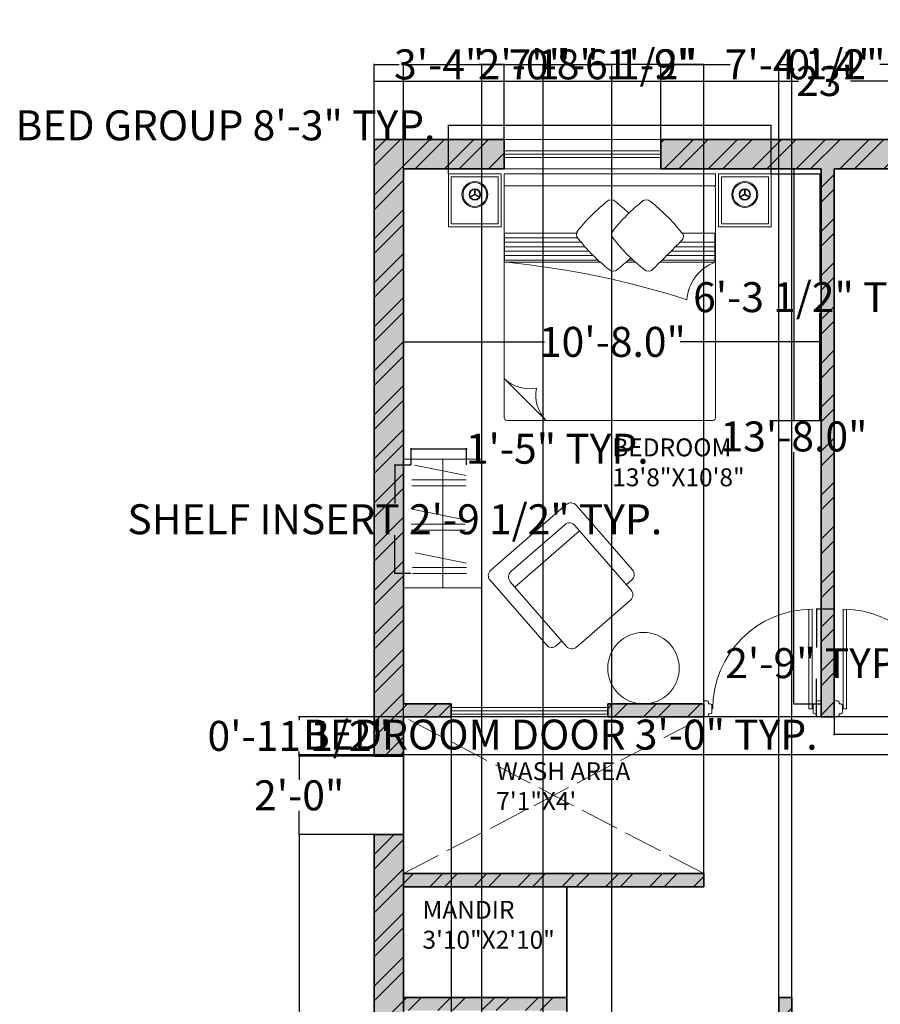
# Model space of a CAD drawing. Units: inches. Extents: x 1086 to 1540, y 3343 to 3848.
# Tile 3 of 8: x 1086 to 1350, y 3547 to 3848. Entities that reach past the tile are written whole.
import ezdxf

# ---------------------------------------------------------------- set-up
doc = ezdxf.new("R2010")
doc.units = ezdxf.units.IN
doc.linetypes.add('ACAD_ISO02W100', pattern=[15, 12, -3])
for name, color, linetype, lineweight in [('00 FURNITURE', 15, 'Continuous', 15), ('A-ANNO-DIMS', 2, 'Continuous', 13), ('A-AREA-IDEN', 7, 'Continuous', 18), ('A-DOOR', 4, 'Continuous', 20), ('A-FLOR-CASE', 8, 'Continuous', 18), ('A-FLOR-OPEN', 8, 'ACAD_ISO02W100', 13), ('A-WALL-PATT', 252, 'Continuous', 9), ('WALL', 7, 'Continuous', 35), ('WINDOW', 160, 'Continuous', 15)]:
    doc.layers.add(name, color=color, linetype=linetype, lineweight=lineweight)
doc.styles.get("Standard").update_dxf_attribs({"font": 'arial.ttf'})
doc.dimstyles.get("Standard").update_dxf_attribs({"dimtxt": 9.18, "dimasz": 0.18, "dimexe": 0.18, "dimexo": 0.0625, "dimgap": 0.09, "dimtad": 0, "dimtih": 1, "dimtoh": 1, "dimdec": 1, "dimzin": 0, "dimdsep": 46, "dimlunit": 3, "dimtxsty": 'Standard', "dimcen": 0.09, "dimadec": 0, "dimazin": 0, "dimtfac": 1, "dimtdec": 1, "dimtofl": 0, "dimtmove": 0, "dimatfit": 3, "dimfxl": 1, "dimtolj": 1, "dimtzin": 0, "dimarcsym": 0})

# ---------------------------------------------------------------- blocks, each defined once
blk = doc.blocks.new('DDD')
at = {"layer": '00 FURNITURE'}
for p, q in [((-12579.77, -15859.53), (-12579.77, -15829.05)), ((-12578.77, -15859.53), (-12578.77, -15829.03)), ((-12612.02, -15857.03), (-12612.02, -15862.03)), ((-12611.02, -15857.03), (-12612.02, -15857.03)), ((-12610.52, -15858.03), (-12610.52, -15857.53)), ((-12578.77, -15859.53), (-12579.77, -15859.53)), ((-12577.52, -15858.03), (-12577.52, -15857.53)), ((-12577.02, -15857.03), (-12576.02, -15857.03)), ((-12576.02, -15857.03), (-12576.02, -15862.03)), ((-12612.02, -15862.03), (-12611.02, -15862.03)), ((-12610.52, -15861.53), (-12610.52, -15861.03)), ((-12577.52, -15861.53), (-12577.52, -15861.03)), ((-12576.02, -15862.03), (-12577.02, -15862.03))]:
    blk.add_line(p, q, dxfattribs=at)
for points in [[(-12610.52, -15861.03), (-12610.02, -15861.03, 0.414214), (-12609.52, -15860.53), (-12609.52, -15858.53, 0.414214), (-12610.02, -15858.03), (-12610.52, -15858.03)], [(-12577.52, -15861.03), (-12578.02, -15861.03, -0.414214), (-12578.52, -15860.53), (-12578.52, -15858.53, -0.414214), (-12578.02, -15858.03), (-12577.52, -15858.03)]]:
    blk.add_lwpolyline(points, format="xyb", dxfattribs=at)
for centre, radius, start, end in [((-12578.77, -15859.53), 30.5, 90, 180), ((-12611.02, -15857.53), 0.5, 0, 90), ((-12577.02, -15857.53), 0.5, 90, 180), ((-12611.02, -15861.53), 0.5, 270, 0), ((-12577.02, -15861.53), 0.5, 180, 270)]:
    blk.add_arc(centre, radius, start, end, dxfattribs=at)
blk = doc.blocks.new('RGWTG')
at = {"layer": '00 FURNITURE'}
for p, q in [((578.23, 3473.51), (577.36, 3475.01)), ((578.23, 3473.58), (577.36, 3472.08)), ((578.36, 3473.58), (577.49, 3475.09)), ((578.36, 3473.51), (577.49, 3472)), ((578.29, 3473.62), (580.03, 3473.62)), ((578.29, 3473.47), (580.03, 3473.47)), ((521.93, 3464.58), (509.03, 3451.68)), ((509.93, 3464.58), (566.4, 3464.58)), ((557.53, 3463.84), (557.53, 3464.49)), ((557.53, 3464.49), (566.4, 3464.49)), ((558.2, 3464.49), (558.2, 3435.82)), ((559.57, 3464.49), (559.57, 3437.25)), ((560.94, 3464.49), (560.94, 3438.58)), ((562.3, 3464.49), (562.3, 3439.83)), ((563.67, 3464.49), (563.67, 3440.99)), ((565.04, 3464.49), (565.04, 3442.08)), ((566.4, 3464.58), (580.98, 3464.58)), ((566.4, 3464.49), (566.4, 3442.08)), ((566.4, 3464.49), (566.4, 3463.84)), ((580.98, 3464.58), (580.98, 3416.72)), ((509.03, 3422.63), (509.03, 3463.68)), ((558.2, 3426.48), (558.2, 3425.04)), ((509.03, 3400.68), (509.03, 3422.63)), ((558.2, 3416.13), (558.2, 3399.95)), ((580.98, 3416.72), (580.98, 3400.68)), ((559.57, 3414.75), (559.57, 3399.95)), ((560.94, 3413.39), (560.94, 3399.95)), ((562.3, 3412.04), (562.3, 3399.95)), ((563.67, 3410.72), (563.67, 3399.95)), ((580.08, 3399.78), (509.93, 3399.78)), ((557.53, 3399.95), (557.53, 3400.6)), ((566.4, 3399.95), (557.53, 3399.95)), ((566.4, 3400.6), (566.4, 3399.95)), ((578.23, 3390.78), (577.36, 3392.29)), ((578.36, 3390.86), (577.49, 3392.36)), ((578.23, 3390.86), (577.36, 3389.36)), ((578.36, 3390.78), (577.49, 3389.28)), ((578.29, 3390.9), (580.03, 3390.9)), ((578.29, 3390.74), (580.03, 3390.74))]:
    blk.add_line(p, q, dxfattribs=at)
for points in [[(568.43, 3465.48), (584.63, 3465.48), (584.63, 3481.68), (568.43, 3481.68)], [(569.33, 3466.38), (583.73, 3466.38), (583.73, 3480.78), (569.33, 3480.78)], [(580.98, 3399.78), (584.63, 3399.78), (584.63, 3464.58), (580.98, 3464.58)], [(568.43, 3398.88), (584.63, 3398.88), (584.63, 3382.68), (568.43, 3382.68)], [(569.33, 3397.98), (583.73, 3397.98), (583.73, 3383.58), (569.33, 3383.58)]]:
    blk.add_lwpolyline(points, close=True, dxfattribs=at)
for points in [[(566.52, 3464.49), (557.53, 3464.49), (557.53, 3435.08)], [(557.53, 3427.21), (557.53, 3424.3)], [(557.53, 3416.82), (557.53, 3399.95), (566.4, 3399.95), (566.4, 3409.94)]]:
    blk.add_lwpolyline(points, dxfattribs=at)
for centre, radius in [((578.29, 3473.54), 3.97), ((578.29, 3473.54), 3.63), ((578.29, 3473.54), 1.74), ((578.29, 3473.54), 1.56), ((578.29, 3390.82), 3.97), ((578.29, 3390.82), 3.63), ((578.29, 3390.82), 1.74), ((578.29, 3390.82), 1.56)]:
    blk.add_circle(centre, radius, dxfattribs=at)
for centre, radius, start, end in [((509.93, 3463.68), 0.9, 90, 180), ((529.65, 3456.88), 10.9, 135.0361, 191.9278), ((290.56, 3490.52), 268.3, 342.2214, 354.2925), ((516.73, 3443.97), 10.9, 78.0722, 134.9639), ((598.15, 3399.01), 54.32, 127.931, 142.069), ((566.05, 3440.57), 1.82, 45, 135), ((533.58, 3399.31), 54.32, 37.931, 52.069), ((556.59, 3431.11), 1.82, 135, 225), ((598.15, 3388.23), 54.32, 127.931, 142.069), ((566.05, 3429.78), 1.82, 45, 135), ((533.58, 3388.53), 54.32, 37.931, 52.069), ((574.84, 3431.77), 1.82, 315, 45), ((597.87, 3463.6), 54.32, 217.931, 224.141), ((533.28, 3463.88), 54.32, 316.32, 322.069), ((574.84, 3420.99), 1.82, 315, 45), ((556.59, 3420.33), 1.82, 135, 225), ((765.33, 3619.75), 290.45, 223.6069, 226.2326), ((533.28, 3453.1), 54.32, 307.931, 322.069), ((565.44, 3411.05), 1.47, 225.9674, 326.8337), ((545.02, 3395.29), 13.35, 20.4224, 85.5825), ((509.93, 3400.68), 0.9, 180, 270), ((580.08, 3400.68), 0.9, 270, 0)]:
    blk.add_arc(centre, radius, start, end, dxfattribs=at)
blk = doc.blocks.new('chair')
at = {"layer": '00 FURNITURE'}
for p, q in [((1373.66, 3525.37), (1373.66, 3527.56)), ((1375.85, 3529.75), (1402.12, 3529.75)), ((1404.31, 3527.56), (1404.31, 3496.9)), ((1371.47, 3525.37), (1397.74, 3525.37)), ((1395.55, 3525.37), (1395.55, 3499.09)), ((1369.28, 3501.28), (1369.28, 3523.18)), ((1399.93, 3523.18), (1399.93, 3501.28)), ((1397.74, 3499.09), (1371.47, 3499.09)), ((1373.66, 3496.9), (1373.66, 3499.09)), ((1402.12, 3494.71), (1375.85, 3494.71))]:
    blk.add_line(p, q, dxfattribs=at)
for centre, start, end in [((1375.85, 3527.56), 90, 180), ((1402.12, 3527.56), 0, 90), ((1371.47, 3523.18), 90, 180), ((1397.74, 3523.18), 0, 90), ((1371.47, 3501.28), 180, 270), ((1397.74, 3501.28), 270, 0), ((1375.85, 3496.9), 180, 270), ((1402.12, 3496.9), 270, 0)]:
    blk.add_arc(centre, 2.19, start, end, dxfattribs=at)
blk = doc.blocks.new('*D12')
at = {"layer": 'A-ANNO-DIMS', "color": 0, "lineweight": -2, "transparency": 16777216}
for p, q in [((1194.74, 3811.63), (1194.74, 3829.64)), ((1194.92, 3829.46), (1324.78, 3829.46)), ((1470.56, 3829.46), (1340.7, 3829.46)), ((1470.74, 3811.63), (1470.74, 3829.64))]:
    blk.add_line(p, q, dxfattribs=at)
at = {"layer": 'A-ANNO-DIMS', "color": 0, "transparency": 16777216}
for points in [[(1194.92, 3829.49), (1194.92, 3829.43), (1194.74, 3829.46)], [(1470.56, 3829.49), (1470.56, 3829.43), (1470.74, 3829.46)]]:
    blk.add_solid(points, dxfattribs=at)
at = {"layer": 'Defpoints', "color": 0, "transparency": 16777216}
for p in [(1470.74, 3829.46), (1194.74, 3811.57), (1470.74, 3811.57)]:
    blk.add_point(p, dxfattribs=at)
at = {"layer": 'A-ANNO-DIMS', "color": 0, "transparency": 16777216, "insert": (1332.74, 3829.46), "char_height": 9.18, "attachment_point": 5}
blk.add_mtext("\\A1;23'", dxfattribs=at)
blk = doc.blocks.new('*D14')
at = {"layer": 'A-ANNO-DIMS', "color": 0, "lineweight": -2, "transparency": 16777216}
for p, q in [((1203.74, 3726.15), (1203.74, 3749.71)), ((1203.92, 3749.53), (1246.97, 3749.53)), ((1331.56, 3749.53), (1288.51, 3749.53)), ((1331.74, 3726.15), (1331.74, 3749.71))]:
    blk.add_line(p, q, dxfattribs=at)
at = {"layer": 'A-ANNO-DIMS', "color": 0, "transparency": 16777216}
for points in [[(1203.92, 3749.56), (1203.92, 3749.5), (1203.74, 3749.53)], [(1331.56, 3749.56), (1331.56, 3749.5), (1331.74, 3749.53)]]:
    blk.add_solid(points, dxfattribs=at)
at = {"layer": 'Defpoints', "color": 0, "transparency": 16777216}
for p in [(1331.74, 3749.53), (1203.74, 3726.09), (1331.74, 3726.09)]:
    blk.add_point(p, dxfattribs=at)
at = {"layer": 'A-ANNO-DIMS', "color": 0, "transparency": 16777216, "insert": (1267.74, 3749.53), "char_height": 9.18, "attachment_point": 5}
blk.add_mtext('\\A1;10\'-8.0"', dxfattribs=at)
blk = doc.blocks.new('*D15')
at = {"layer": 'A-ANNO-DIMS', "color": 0, "lineweight": -2, "transparency": 16777216}
for p, q in [((1331.68, 3802.57), (1323.22, 3802.57)), ((1323.4, 3802.39), (1323.4, 3725.33)), ((1323.4, 3638.7), (1323.4, 3715.77)), ((1331.68, 3638.52), (1323.22, 3638.52))]:
    blk.add_line(p, q, dxfattribs=at)
at = {"layer": 'A-ANNO-DIMS', "color": 0, "transparency": 16777216}
for points in [[(1323.37, 3802.39), (1323.43, 3802.39), (1323.4, 3802.57)], [(1323.37, 3638.7), (1323.43, 3638.7), (1323.4, 3638.52)]]:
    blk.add_solid(points, dxfattribs=at)
at = {"layer": 'Defpoints', "color": 0, "transparency": 16777216}
for p in [(1331.74, 3802.57), (1323.4, 3638.52), (1331.74, 3638.52)]:
    blk.add_point(p, dxfattribs=at)
at = {"layer": 'A-ANNO-DIMS', "color": 0, "transparency": 16777216, "insert": (1323.4, 3720.55), "char_height": 9.18, "attachment_point": 5}
blk.add_mtext('\\A1;13\'-8.0"', dxfattribs=at)
blk = doc.blocks.new('WIN-GLAZING-48IN')
for p, q in [((48, 1), (0, 1)), ((48, 0), (0, 0)), ((48, -1), (0, -1))]:
    blk.add_line(p, q)
blk = doc.blocks.new('BOOKCASE-FRAME')
for p, q in [((24, 39.45), (0, 39.45)), ((12, 39.45), (12, 0)), ((24, 0), (24, 39.45)), ((0, 0), (24, 0))]:
    blk.add_line(p, q)
blk = doc.blocks.new('BOOKCASE-CONTENTS')
for p, q in [((0.85, 6.37), (16.59, 3.17)), ((0, 1.86), (16.59, 1.86)), ((0, 0), (16.59, 0)), ((0.59, -7.26), (16.34, -10.46)), ((-0.25, -11.76), (16.34, -11.76)), ((-0.25, -13.62), (16.34, -13.62)), ((0.99, -20.52), (16.73, -23.72)), ((0.14, -25.02), (16.73, -25.02)), ((0.14, -26.89), (16.73, -26.89))]:
    blk.add_line(p, q)
blk = doc.blocks.new('TABLE-ROUND-SIDE')
blk.add_circle((0, 0), 10.95)
blk = doc.blocks.new('*D21')
at = {"layer": 'A-ANNO-DIMS', "color": 0, "lineweight": -2, "transparency": 16777216}
for p, q in [((1217.45, 3815.88), (1217.27, 3815.88)), ((1217.45, 3801.1), (1217.45, 3816.06)), ((1316.27, 3815.88), (1217.63, 3815.88)), ((1316.45, 3801.1), (1316.45, 3816.06))]:
    blk.add_line(p, q, dxfattribs=at)
at = {"layer": 'A-ANNO-DIMS', "color": 0, "transparency": 16777216}
for points in [[(1217.63, 3815.91), (1217.63, 3815.85), (1217.45, 3815.88)], [(1316.27, 3815.91), (1316.27, 3815.85), (1316.45, 3815.88)]]:
    blk.add_solid(points, dxfattribs=at)
at = {"layer": 'Defpoints', "color": 0, "transparency": 16777216}
for p in [(1217.45, 3815.88), (1217.45, 3801.03), (1316.45, 3801.03)]:
    blk.add_point(p, dxfattribs=at)
at = {"layer": 'A-ANNO-DIMS', "color": 0, "transparency": 16777216, "insert": (1149.14, 3815.88), "char_height": 9.18, "attachment_point": 5}
blk.add_mtext('\\A1;BED GROUP 8\'-3" TYP.', dxfattribs=at)
blk = doc.blocks.new('*D22')
at = {"layer": 'A-ANNO-DIMS', "color": 0, "lineweight": -2, "transparency": 16777216}
for p, q in [((1316.51, 3801.03), (1331.48, 3801.03)), ((1331.3, 3800.85), (1331.3, 3768.07)), ((1331.3, 3725.61), (1331.3, 3758.39)), ((1316.51, 3725.43), (1331.48, 3725.43))]:
    blk.add_line(p, q, dxfattribs=at)
at = {"layer": 'A-ANNO-DIMS', "color": 0, "transparency": 16777216}
for points in [[(1331.27, 3800.85), (1331.33, 3800.85), (1331.3, 3801.03)], [(1331.27, 3725.61), (1331.33, 3725.61), (1331.3, 3725.43)]]:
    blk.add_solid(points, dxfattribs=at)
at = {"layer": 'Defpoints', "color": 0, "transparency": 16777216}
for p in [(1316.45, 3801.03), (1331.3, 3801.03), (1316.45, 3725.43)]:
    blk.add_point(p, dxfattribs=at)
at = {"layer": 'A-ANNO-DIMS', "color": 0, "transparency": 16777216, "insert": (1331.3, 3763.23), "char_height": 9.18, "attachment_point": 5}
blk.add_mtext('\\A1;6\'-3 1/2" TYP.', dxfattribs=at)
blk = doc.blocks.new('*D25')
at = {"layer": 'A-ANNO-DIMS', "color": 0, "lineweight": -2, "transparency": 16777216}
for p, q in [((1335.74, 3634.51), (1335.74, 3628.99)), ((1371.74, 3634.51), (1371.74, 3628.99)), ((1335.74, 3629.17), (1335.56, 3629.17)), ((1371.56, 3629.17), (1335.92, 3629.17))]:
    blk.add_line(p, q, dxfattribs=at)
at = {"layer": 'A-ANNO-DIMS', "color": 0, "transparency": 16777216}
for points in [[(1335.92, 3629.2), (1335.92, 3629.14), (1335.74, 3629.17)], [(1371.56, 3629.2), (1371.56, 3629.14), (1371.74, 3629.17)]]:
    blk.add_solid(points, dxfattribs=at)
at = {"layer": 'Defpoints', "color": 0, "transparency": 16777216}
for p in [(1335.74, 3634.57), (1371.74, 3634.57), (1335.74, 3629.17)]:
    blk.add_point(p, dxfattribs=at)
at = {"layer": 'A-ANNO-DIMS', "color": 0, "transparency": 16777216, "insert": (1251.76, 3629.17), "char_height": 9.18, "attachment_point": 5}
blk.add_mtext('\\A1;BEDROOM DOOR 3\'-0" TYP.', dxfattribs=at)
blk = doc.blocks.new('*D26')
at = {"layer": 'A-ANNO-DIMS', "color": 0, "lineweight": -2, "transparency": 16777216}
for p, q in [((1335.68, 3667.57), (1330.16, 3667.57)), ((1330.34, 3667.39), (1330.34, 3655.85)), ((1330.34, 3634.75), (1330.34, 3646.29)), ((1335.68, 3634.57), (1330.16, 3634.57))]:
    blk.add_line(p, q, dxfattribs=at)
at = {"layer": 'A-ANNO-DIMS', "color": 0, "transparency": 16777216}
for points in [[(1330.31, 3667.39), (1330.37, 3667.39), (1330.34, 3667.57)], [(1330.31, 3634.75), (1330.37, 3634.75), (1330.34, 3634.57)]]:
    blk.add_solid(points, dxfattribs=at)
at = {"layer": 'Defpoints', "color": 0, "transparency": 16777216}
for p in [(1330.34, 3667.57), (1335.74, 3667.57), (1335.74, 3634.57)]:
    blk.add_point(p, dxfattribs=at)
at = {"layer": 'A-ANNO-DIMS', "color": 0, "transparency": 16777216, "insert": (1330.34, 3651.07), "char_height": 9.18, "attachment_point": 5}
blk.add_mtext('\\A1;2\'-9" TYP.', dxfattribs=at)
blk = doc.blocks.new('*D33')
at = {"layer": 'A-ANNO-DIMS', "color": 0, "lineweight": -2, "transparency": 16777216}
for p, q in [((1205.97, 3711.79), (1200.86, 3711.79)), ((1201.04, 3711.61), (1201.04, 3700)), ((1201.04, 3678.72), (1201.04, 3690.33)), ((1205.97, 3678.54), (1200.86, 3678.54))]:
    blk.add_line(p, q, dxfattribs=at)
at = {"layer": 'A-ANNO-DIMS', "color": 0, "transparency": 16777216}
for points in [[(1201.01, 3711.61), (1201.07, 3711.61), (1201.04, 3711.79)], [(1201.01, 3678.72), (1201.07, 3678.72), (1201.04, 3678.54)]]:
    blk.add_solid(points, dxfattribs=at)
at = {"layer": 'Defpoints', "color": 0, "transparency": 16777216}
for p in [(1201.04, 3711.79), (1206.03, 3711.79), (1206.03, 3678.54)]:
    blk.add_point(p, dxfattribs=at)
at = {"layer": 'A-ANNO-DIMS', "color": 0, "transparency": 16777216, "insert": (1201.04, 3695.16), "char_height": 9.18, "attachment_point": 5}
blk.add_mtext('\\A1;SHELF INSERT 2\'-9 1/2" TYP.', dxfattribs=at)
blk = doc.blocks.new('*D34')
at = {"layer": 'A-ANNO-DIMS', "color": 0, "lineweight": -2, "transparency": 16777216}
for p, q in [((1206.03, 3711.86), (1206.03, 3716.96)), ((1206.21, 3716.78), (1222.84, 3716.78)), ((1223.02, 3711.86), (1223.02, 3716.96)), ((1223.02, 3716.78), (1223.2, 3716.78))]:
    blk.add_line(p, q, dxfattribs=at)
at = {"layer": 'A-ANNO-DIMS', "color": 0, "transparency": 16777216}
for points in [[(1206.21, 3716.81), (1206.21, 3716.75), (1206.03, 3716.78)], [(1222.84, 3716.81), (1222.84, 3716.75), (1223.02, 3716.78)]]:
    blk.add_solid(points, dxfattribs=at)
at = {"layer": 'Defpoints', "color": 0, "transparency": 16777216}
for p in [(1223.02, 3716.78), (1206.03, 3711.79), (1223.02, 3711.79)]:
    blk.add_point(p, dxfattribs=at)
at = {"layer": 'A-ANNO-DIMS', "color": 0, "transparency": 16777216, "insert": (1250.83, 3716.78), "char_height": 9.18, "attachment_point": 5}
blk.add_mtext('\\A1;1\'-5" TYP.', dxfattribs=at)
blk = doc.blocks.new('*D47')
at = {"layer": 'A-ANNO-DIMS', "color": 0, "lineweight": -2, "transparency": 16777216}
for p, q in [((1194.74, 3811.63), (1194.74, 3834.75)), ((1194.92, 3834.57), (1202.36, 3834.57)), ((1234.37, 3834.57), (1226.93, 3834.57)), ((1234.55, 3811.63), (1234.55, 3834.75))]:
    blk.add_line(p, q, dxfattribs=at)
at = {"layer": 'A-ANNO-DIMS', "color": 0, "transparency": 16777216}
for points in [[(1194.92, 3834.6), (1194.92, 3834.54), (1194.74, 3834.57)], [(1234.37, 3834.6), (1234.37, 3834.54), (1234.55, 3834.57)]]:
    blk.add_solid(points, dxfattribs=at)
at = {"layer": 'Defpoints', "color": 0, "transparency": 16777216}
for p in [(1234.55, 3834.57), (1194.74, 3811.57), (1234.55, 3811.57)]:
    blk.add_point(p, dxfattribs=at)
at = {"layer": 'A-ANNO-DIMS', "color": 0, "transparency": 16777216, "insert": (1214.65, 3834.57), "char_height": 9.18, "attachment_point": 5}
blk.add_mtext('\\A1;3\'-4"', dxfattribs=at)
blk = doc.blocks.new('*D48')
at = {"layer": 'A-ANNO-DIMS', "color": 0, "lineweight": -2, "transparency": 16777216}
for p, q in [((1282.55, 3811.63), (1282.55, 3834.75)), ((1282.73, 3834.57), (1303.86, 3834.57)), ((1370.88, 3834.57), (1349.75, 3834.57)), ((1371.06, 3811.63), (1371.06, 3834.75))]:
    blk.add_line(p, q, dxfattribs=at)
at = {"layer": 'A-ANNO-DIMS', "color": 0, "transparency": 16777216}
for points in [[(1282.73, 3834.6), (1282.73, 3834.54), (1282.55, 3834.57)], [(1370.88, 3834.6), (1370.88, 3834.54), (1371.06, 3834.57)]]:
    blk.add_solid(points, dxfattribs=at)
at = {"layer": 'Defpoints', "color": 0, "transparency": 16777216}
for p in [(1371.06, 3834.57), (1282.55, 3811.57), (1371.06, 3811.57)]:
    blk.add_point(p, dxfattribs=at)
at = {"layer": 'A-ANNO-DIMS', "color": 0, "transparency": 16777216, "insert": (1326.8, 3834.57), "char_height": 9.18, "attachment_point": 5}
blk.add_mtext('\\A1;7\'-4 1/2"', dxfattribs=at)
blk = doc.blocks.new('*D51')
at = {"layer": 'A-ANNO-DIMS', "color": 0, "lineweight": -2, "transparency": 16777216}
for p, q in [((1318.74, 3548.63), (1318.74, 3834.75)), ((1318.92, 3834.57), (1322.56, 3834.57)), ((1322.74, 3548.63), (1322.74, 3834.75)), ((1322.74, 3834.57), (1322.92, 3834.57))]:
    blk.add_line(p, q, dxfattribs=at)
at = {"layer": 'A-ANNO-DIMS', "color": 0, "transparency": 16777216}
for points in [[(1318.92, 3834.6), (1318.92, 3834.54), (1318.74, 3834.57)], [(1322.56, 3834.6), (1322.56, 3834.54), (1322.74, 3834.57)]]:
    blk.add_solid(points, dxfattribs=at)
at = {"layer": 'Defpoints', "color": 0, "transparency": 16777216}
for p in [(1322.74, 3834.57), (1318.74, 3548.57), (1322.74, 3548.57)]:
    blk.add_point(p, dxfattribs=at)
at = {"layer": 'A-ANNO-DIMS', "color": 0, "transparency": 16777216, "insert": (1335.21, 3834.57), "char_height": 9.18, "attachment_point": 5}
blk.add_mtext('\\A1;0\'-4"', dxfattribs=at)
blk = doc.blocks.new('*D52')
at = {"layer": 'A-ANNO-DIMS', "color": 0, "lineweight": -2, "transparency": 16777216}
for p, q in [((1194.68, 3598.57), (1171.56, 3598.57)), ((1171.74, 3598.39), (1171.74, 3493.85)), ((1171.74, 3379.75), (1171.74, 3484.29)), ((1194.68, 3379.57), (1171.56, 3379.57))]:
    blk.add_line(p, q, dxfattribs=at)
at = {"layer": 'A-ANNO-DIMS', "color": 0, "transparency": 16777216}
for points in [[(1171.71, 3598.39), (1171.77, 3598.39), (1171.74, 3598.57)], [(1171.71, 3379.75), (1171.77, 3379.75), (1171.74, 3379.57)]]:
    blk.add_solid(points, dxfattribs=at)
at = {"layer": 'Defpoints', "color": 0, "transparency": 16777216}
for p in [(1171.74, 3598.57), (1194.74, 3598.57), (1194.74, 3379.57)]:
    blk.add_point(p, dxfattribs=at)
at = {"layer": 'A-ANNO-DIMS', "color": 0, "transparency": 16777216, "insert": (1171.74, 3489.07), "char_height": 9.18, "attachment_point": 5}
blk.add_mtext('\\A1;18\'-3"', dxfattribs=at)
blk = doc.blocks.new('*D53')
at = {"layer": 'A-ANNO-DIMS', "color": 0, "lineweight": -2, "transparency": 16777216}
for p, q in [((1194.68, 3622.57), (1171.56, 3622.57)), ((1171.74, 3622.39), (1171.74, 3615.35)), ((1171.74, 3598.75), (1171.74, 3605.79)), ((1194.68, 3598.57), (1171.56, 3598.57))]:
    blk.add_line(p, q, dxfattribs=at)
at = {"layer": 'A-ANNO-DIMS', "color": 0, "transparency": 16777216}
for points in [[(1171.71, 3622.39), (1171.77, 3622.39), (1171.74, 3622.57)], [(1171.71, 3598.75), (1171.77, 3598.75), (1171.74, 3598.57)]]:
    blk.add_solid(points, dxfattribs=at)
at = {"layer": 'Defpoints', "color": 0, "transparency": 16777216}
for p in [(1171.74, 3622.57), (1194.74, 3622.57), (1194.74, 3598.57)]:
    blk.add_point(p, dxfattribs=at)
at = {"layer": 'A-ANNO-DIMS', "color": 0, "transparency": 16777216, "insert": (1171.74, 3610.57), "char_height": 9.18, "attachment_point": 5}
blk.add_mtext('\\A1;2\'-0"', dxfattribs=at)
blk = doc.blocks.new('*D55')
at = {"layer": 'A-ANNO-DIMS', "color": 0, "lineweight": -2, "transparency": 16777216}
for p, q in [((1203.74, 3634.51), (1203.74, 3356.39)), ((1218.33, 3634.51), (1218.33, 3356.39)), ((1203.92, 3356.57), (1218.15, 3356.57)), ((1218.33, 3356.57), (1218.51, 3356.57))]:
    blk.add_line(p, q, dxfattribs=at)
at = {"layer": 'A-ANNO-DIMS', "color": 0, "transparency": 16777216}
for points in [[(1203.92, 3356.6), (1203.92, 3356.54), (1203.74, 3356.57)], [(1218.15, 3356.6), (1218.15, 3356.54), (1218.33, 3356.57)]]:
    blk.add_solid(points, dxfattribs=at)
at = {"layer": 'Defpoints', "color": 0, "transparency": 16777216}
for p in [(1203.74, 3634.57), (1218.33, 3634.57), (1218.33, 3356.57)]:
    blk.add_point(p, dxfattribs=at)
at = {"layer": 'A-ANNO-DIMS', "color": 0, "transparency": 16777216, "insert": (1241.07, 3356.57), "char_height": 9.18, "attachment_point": 5}
blk.add_mtext('\\A1;1\'-2 1/2"', dxfattribs=at)
blk = doc.blocks.new('*D56')
at = {"layer": 'A-ANNO-DIMS', "color": 0, "lineweight": -2, "transparency": 16777216}
for p, q in [((1203.74, 3544.63), (1203.74, 3834.75)), ((1203.92, 3834.57), (1227.56, 3834.57)), ((1227.74, 3544.63), (1227.74, 3834.75)), ((1227.74, 3834.57), (1227.92, 3834.57))]:
    blk.add_line(p, q, dxfattribs=at)
at = {"layer": 'A-ANNO-DIMS', "color": 0, "transparency": 16777216}
for points in [[(1203.92, 3834.6), (1203.92, 3834.54), (1203.74, 3834.57)], [(1227.56, 3834.6), (1227.56, 3834.54), (1227.74, 3834.57)]]:
    blk.add_solid(points, dxfattribs=at)
at = {"layer": 'Defpoints', "color": 0, "transparency": 16777216}
for p in [(1227.74, 3834.57), (1203.74, 3544.57), (1227.74, 3544.57)]:
    blk.add_point(p, dxfattribs=at)
at = {"layer": 'A-ANNO-DIMS', "color": 0, "transparency": 16777216, "insert": (1240.29, 3834.57), "char_height": 9.18, "attachment_point": 5}
blk.add_mtext('\\A1;2\'-0"', dxfattribs=at)
blk = doc.blocks.new('*D58')
at = {"layer": 'A-ANNO-DIMS', "color": 0, "lineweight": -2, "transparency": 16777216}
for p, q in [((1246.48, 3479.63), (1246.48, 3834.75)), ((1246.66, 3834.57), (1267.34, 3834.57)), ((1267.52, 3479.63), (1267.52, 3834.75)), ((1267.52, 3834.57), (1267.7, 3834.57))]:
    blk.add_line(p, q, dxfattribs=at)
at = {"layer": 'A-ANNO-DIMS', "color": 0, "transparency": 16777216}
for points in [[(1246.66, 3834.6), (1246.66, 3834.54), (1246.48, 3834.57)], [(1267.34, 3834.6), (1267.34, 3834.54), (1267.52, 3834.57)]]:
    blk.add_solid(points, dxfattribs=at)
at = {"layer": 'Defpoints', "color": 0, "transparency": 16777216}
for p in [(1267.52, 3834.57), (1246.48, 3479.57), (1267.52, 3479.57)]:
    blk.add_point(p, dxfattribs=at)
at = {"layer": 'A-ANNO-DIMS', "color": 0, "transparency": 16777216, "insert": (1279.55, 3834.57), "char_height": 9.18, "attachment_point": 5}
blk.add_mtext('\\A1;1\'-9"', dxfattribs=at)
blk = doc.blocks.new('*D60')
at = {"layer": 'A-ANNO-DIMS', "color": 0, "lineweight": -2, "transparency": 16777216}
for p, q in [((1227.74, 3479.63), (1227.74, 3834.75)), ((1227.92, 3834.57), (1246.3, 3834.57)), ((1246.48, 3479.63), (1246.48, 3834.75)), ((1246.48, 3834.57), (1246.66, 3834.57))]:
    blk.add_line(p, q, dxfattribs=at)
at = {"layer": 'A-ANNO-DIMS', "color": 0, "transparency": 16777216}
for points in [[(1227.92, 3834.6), (1227.92, 3834.54), (1227.74, 3834.57)], [(1246.3, 3834.6), (1246.3, 3834.54), (1246.48, 3834.57)]]:
    blk.add_solid(points, dxfattribs=at)
at = {"layer": 'Defpoints', "color": 0, "transparency": 16777216}
for p in [(1246.48, 3834.57), (1227.74, 3479.57), (1246.48, 3479.57)]:
    blk.add_point(p, dxfattribs=at)
at = {"layer": 'A-ANNO-DIMS', "color": 0, "transparency": 16777216, "insert": (1269.22, 3834.57), "char_height": 9.18, "attachment_point": 5}
blk.add_mtext('\\A1;1\'-6 1/2"', dxfattribs=at)
blk = doc.blocks.new('*D69')
at = {"layer": 'A-ANNO-DIMS', "color": 0, "lineweight": -2, "transparency": 16777216}
for p, q in [((1421.68, 3634.57), (1171.56, 3634.57)), ((1171.74, 3634.39), (1171.74, 3633.62)), ((1171.74, 3623.18), (1171.74, 3623.95)), ((1420.44, 3623), (1171.56, 3623))]:
    blk.add_line(p, q, dxfattribs=at)
at = {"layer": 'A-ANNO-DIMS', "color": 0, "transparency": 16777216}
for points in [[(1171.71, 3634.39), (1171.77, 3634.39), (1171.74, 3634.57)], [(1171.71, 3623.18), (1171.77, 3623.18), (1171.74, 3623)]]:
    blk.add_solid(points, dxfattribs=at)
at = {"layer": 'Defpoints', "color": 0, "transparency": 16777216}
for p in [(1421.74, 3634.57), (1171.74, 3623), (1420.5, 3623)]:
    blk.add_point(p, dxfattribs=at)
at = {"layer": 'A-ANNO-DIMS', "color": 0, "transparency": 16777216, "insert": (1171.74, 3628.78), "char_height": 9.18, "attachment_point": 5}
blk.add_mtext('\\A1;0\'-11 1/2"', dxfattribs=at)
blk = doc.blocks.new('*D72')
at = {"layer": 'A-ANNO-DIMS', "color": 0, "lineweight": -2, "transparency": 16777216}
for p, q in [((1318.74, 3548.51), (1318.74, 3356.39)), ((1253.74, 3544.51), (1253.74, 3356.39)), ((1253.92, 3356.57), (1273.95, 3356.57)), ((1318.56, 3356.57), (1298.53, 3356.57))]:
    blk.add_line(p, q, dxfattribs=at)
at = {"layer": 'A-ANNO-DIMS', "color": 0, "transparency": 16777216}
for points in [[(1253.92, 3356.6), (1253.92, 3356.54), (1253.74, 3356.57)], [(1318.56, 3356.6), (1318.56, 3356.54), (1318.74, 3356.57)]]:
    blk.add_solid(points, dxfattribs=at)
at = {"layer": 'Defpoints', "color": 0, "transparency": 16777216}
for p in [(1318.74, 3548.57), (1253.74, 3544.57), (1318.74, 3356.57)]:
    blk.add_point(p, dxfattribs=at)
at = {"layer": 'A-ANNO-DIMS', "color": 0, "transparency": 16777216, "insert": (1286.24, 3356.57), "char_height": 9.18, "attachment_point": 5}
blk.add_mtext('\\A1;5\'-5"', dxfattribs=at)
blk = doc.blocks.new('*D74')
at = {"layer": 'A-ANNO-DIMS', "color": 0, "lineweight": -2, "transparency": 16777216}
for p, q in [((1203.74, 3586.63), (1203.74, 3834.75)), ((1203.92, 3834.57), (1237.49, 3834.57)), ((1295.56, 3834.57), (1261.99, 3834.57)), ((1295.74, 3586.63), (1295.74, 3834.75))]:
    blk.add_line(p, q, dxfattribs=at)
at = {"layer": 'A-ANNO-DIMS', "color": 0, "transparency": 16777216}
for points in [[(1203.92, 3834.6), (1203.92, 3834.54), (1203.74, 3834.57)], [(1295.56, 3834.6), (1295.56, 3834.54), (1295.74, 3834.57)]]:
    blk.add_solid(points, dxfattribs=at)
at = {"layer": 'Defpoints', "color": 0, "transparency": 16777216}
for p in [(1295.74, 3834.57), (1203.74, 3586.57), (1295.74, 3586.57)]:
    blk.add_point(p, dxfattribs=at)
at = {"layer": 'A-ANNO-DIMS', "color": 0, "transparency": 16777216, "insert": (1249.74, 3834.57), "char_height": 9.18, "attachment_point": 5}
blk.add_mtext('\\A1;7\'-8"', dxfattribs=at)

msp = doc.modelspace()

# ---------------------------------------------------------------- hatches: boundary and pattern name
at = {"layer": 'A-WALL-PATT'}
h = msp.add_hatch(dxfattribs=at)
h.set_pattern_fill('ANSI32', color=256)
h.paths.add_polyline_path([(1234.55, 3811.57), (1234.55, 3811.57), (1194.74, 3811.57), (1194.74, 3622.57), (1203.74, 3622.57), (1203.74, 3634.57), (1218.33, 3634.57), (1218.33, 3638.57), (1203.74, 3638.57), (1203.74, 3802.57), (1234.55, 3802.57)])
h.paths.add_polyline_path([(1371.06, 3811.57), (1371.06, 3811.57), (1282.55, 3811.57), (1282.55, 3802.57), (1331.74, 3802.57), (1331.74, 3634.57), (1335.74, 3634.57), (1335.74, 3639.57), (1335.74, 3802.57), (1371.06, 3802.57)])
h.paths.add_polyline_path([(1470.74, 3811.57), (1419.06, 3811.57), (1419.06, 3802.57), (1461.74, 3802.57), (1461.74, 3638.57), (1461.74, 3548.57), (1425.74, 3548.57), (1425.74, 3582.21), (1421.74, 3582.21), (1421.74, 3548.57), (1376.74, 3548.57), (1376.74, 3602.57), (1373.71, 3602.57), (1372.74, 3602.57), (1372.74, 3544.57), (1461.74, 3544.57), (1461.74, 3379.57), (1470.74, 3379.57)])
h.paths.add_polyline_path([(1203.74, 3582.57), (1295.74, 3582.57), (1295.74, 3586.57), (1203.74, 3586.57), (1203.74, 3598.57), (1194.74, 3598.57), (1194.74, 3379.57), (1326.74, 3379.57), (1326.74, 3388.57), (1322.74, 3388.57), (1203.74, 3388.57), (1203.74, 3451.57), (1234.74, 3451.57), (1234.74, 3455.57), (1203.74, 3455.57), (1203.74, 3479.57), (1203.74, 3544.57), (1227.74, 3544.57), (1253.74, 3544.57), (1253.74, 3548.57), (1203.74, 3548.57)])
h.paths.add_polyline_path([(1461.74, 3638.57), (1371.74, 3638.57), (1371.74, 3634.57), (1372.74, 3634.57), (1372.74, 3632.57), (1376.74, 3632.57), (1376.74, 3634.57), (1421.74, 3634.57), (1421.74, 3606.21), (1425.74, 3606.21), (1425.74, 3634.57), (1461.74, 3634.57)])
h.paths.add_polyline_path([(1295.74, 3638.57), (1266.33, 3638.57), (1266.33, 3634.57), (1292.74, 3634.57), (1295.74, 3634.57)])
h.paths.add_polyline_path([(1322.74, 3548.57), (1318.74, 3548.57), (1318.74, 3455.57), (1282.74, 3455.57), (1282.74, 3451.57), (1318.74, 3451.57), (1318.74, 3420.07), (1322.74, 3420.07)], flags=17)
at = {"layer": 'A-WALL-PATT', "transparency": 33554559}
h = msp.add_hatch(color=256, dxfattribs=at)
h.dxf.hatch_style = 1
h.paths.add_polyline_path([(1234.55, 3811.57), (1234.55, 3811.57), (1194.74, 3811.57), (1194.74, 3622.57), (1203.74, 3622.57), (1203.74, 3634.57), (1218.33, 3634.57), (1218.33, 3638.57), (1203.74, 3638.57), (1203.74, 3802.57), (1234.55, 3802.57)])
h.paths.add_polyline_path([(1371.06, 3811.57), (1371.06, 3811.57), (1282.55, 3811.57), (1282.55, 3802.57), (1331.74, 3802.57), (1331.74, 3634.57), (1335.74, 3634.57), (1335.74, 3639.57), (1335.74, 3802.57), (1371.06, 3802.57)])
h.paths.add_polyline_path([(1470.74, 3811.57), (1419.06, 3811.57), (1419.06, 3802.57), (1461.74, 3802.57), (1461.74, 3638.57), (1461.74, 3548.57), (1425.74, 3548.57), (1425.74, 3582.21), (1421.74, 3582.21), (1421.74, 3548.57), (1376.74, 3548.57), (1376.74, 3602.57), (1372.74, 3602.57), (1372.74, 3544.57), (1461.74, 3544.57), (1461.74, 3379.57), (1470.74, 3379.57)])
h.paths.add_polyline_path([(1203.74, 3544.57), (1227.74, 3544.57), (1253.74, 3544.57), (1253.74, 3548.57), (1203.74, 3548.57), (1203.74, 3582.57), (1295.74, 3582.57), (1295.74, 3586.57), (1203.74, 3586.57), (1203.74, 3598.57), (1194.74, 3598.57), (1194.74, 3379.57), (1326.74, 3379.57), (1326.74, 3388.57), (1322.74, 3388.57), (1203.74, 3388.57), (1203.74, 3451.57), (1234.74, 3451.57), (1234.74, 3455.57), (1203.74, 3455.57)])
h.paths.add_polyline_path([(1413.74, 3388.57), (1413.74, 3388.57), (1374.74, 3388.57), (1374.74, 3383.18), (1374.74, 3383.18), (1374.74, 3379.57), (1413.74, 3379.57)], flags=17)
h.paths.add_polyline_path([(1322.74, 3548.57), (1318.74, 3548.57), (1318.74, 3455.57), (1282.74, 3455.57), (1282.74, 3451.57), (1318.74, 3451.57), (1318.74, 3420.07), (1322.74, 3420.07)], flags=17)
h.paths.add_polyline_path([(1295.74, 3638.57), (1266.33, 3638.57), (1266.33, 3634.57), (1292.74, 3634.57), (1295.74, 3634.57)])
h.paths.add_polyline_path([(1461.74, 3638.57), (1371.74, 3638.57), (1371.74, 3634.57), (1372.74, 3634.57), (1372.74, 3632.57), (1376.74, 3632.57), (1376.74, 3634.57), (1421.74, 3634.57), (1421.74, 3606.21), (1425.74, 3606.21), (1425.74, 3634.57), (1461.74, 3634.57)])

# ---------------------------------------------------------------- linework, layer by layer
at = {"layer": 'A-FLOR-OPEN'}
for p, q in [((1203.74, 3586.57), (1296.74, 3635.07)), ((1295.74, 3586.57), (1203.74, 3634.57))]:
    msp.add_line(p, q, dxfattribs=at)
at = {"layer": 'WALL'}
for p, q in [((1194.74, 3811.57), (1234.55, 3811.57)), ((1194.74, 3622.57), (1194.74, 3811.57)), ((1234.55, 3802.57), (1234.55, 3811.57)), ((1282.55, 3802.57), (1282.55, 3811.57)), ((1282.55, 3811.57), (1371.06, 3811.57)), ((1203.74, 3802.57), (1234.55, 3802.57)), ((1203.74, 3638.57), (1203.74, 3802.57)), ((1282.55, 3802.57), (1331.74, 3802.57)), ((1331.74, 3634.57), (1331.74, 3802.57)), ((1335.74, 3634.57), (1335.74, 3802.57)), ((1335.74, 3802.57), (1371.06, 3802.57)), ((1203.74, 3638.57), (1218.33, 3638.57)), ((1218.33, 3634.57), (1218.33, 3638.57)), ((1266.33, 3634.57), (1266.33, 3638.57)), ((1266.33, 3638.57), (1295.74, 3638.57)), ((1295.74, 3634.57), (1295.74, 3638.57)), ((1203.74, 3634.57), (1218.33, 3634.57)), ((1203.74, 3622.57), (1203.74, 3634.57)), ((1266.33, 3634.57), (1292.74, 3634.57)), ((1292.74, 3634.57), (1295.74, 3634.57)), ((1331.74, 3634.57), (1335.74, 3634.57)), ((1203.74, 3622.57), (1194.74, 3622.57)), ((1194.74, 3379.57), (1194.74, 3598.57)), ((1203.74, 3598.57), (1194.74, 3598.57)), ((1203.74, 3586.57), (1203.74, 3598.57)), ((1203.74, 3586.57), (1295.74, 3586.57)), ((1295.74, 3586.57), (1295.74, 3582.57)), ((1203.74, 3582.57), (1295.74, 3582.57)), ((1203.74, 3548.57), (1203.74, 3582.57)), ((1253.74, 3544.57), (1253.74, 3582.57)), ((1203.74, 3548.57), (1253.74, 3548.57)), ((1318.74, 3548.57), (1322.74, 3548.57)), ((1318.74, 3455.57), (1318.74, 3548.57)), ((1322.74, 3420.07), (1322.74, 3548.57))]:
    msp.add_line(p, q, dxfattribs=at)
at = {"layer": 'WINDOW'}
for p, q in [((1282.55, 3811.57), (1234.55, 3811.57)), ((1234.55, 3802.57), (1282.55, 3802.57))]:
    msp.add_line(p, q, dxfattribs=at)

# ---------------------------------------------------------------- block references
at = {"layer": '00 FURNITURE'}
for name, p, rotation in [('RGWTG', (4699.13, 3216.4), 89.99999999999999), ('chair', (4813.2, 4936.41), 131.0387198642023)]:
    msp.add_blockref(name, p, dxfattribs=dict(at, rotation=rotation))
msp.add_blockref('TABLE-ROUND-SIDE', (1277.28, 3649.52), dxfattribs=at)
at = {"layer": 'A-DOOR'}
msp.add_blockref('DDD', (13907.76, 19496.6), dxfattribs=at)
at = {"layer": 'A-DOOR', "xscale": -1}
msp.add_blockref('DDD', (-11240.28, 19496.6), dxfattribs=at)
at = {"layer": 'A-FLOR-CASE'}
for name, p in [('BOOKCASE-FRAME', (1203.74, 3674.16)), ('BOOKCASE-CONTENTS', (1206.28, 3705.42))]:
    msp.add_blockref(name, p, dxfattribs=at)
at = {"layer": 'WINDOW'}
for p in [(1234.55, 3807.07), (1218.29, 3636.48)]:
    msp.add_blockref('WIN-GLAZING-48IN', p, dxfattribs=at)

# ---------------------------------------------------------------- texts
at = {"layer": 'A-AREA-IDEN', "char_height": 8, "attachment_point": 1}
for s, insert in [('{\\H0.6875x;BEDROOM\\P13\'8"X10\'8"\\H1.1818x; }  ', (1267.7, 3719.94)), ('{\\H0.6875x;WASH AREA\\P7\'1"X4\'\\H1.1818x; }  ', (1232.15, 3620.71)), ('{\\H0.6875x;MANDIR\\P3\'10"X2\'10"} ', (1209.52, 3578.22))]:
    msp.add_mtext_dynamic_manual_height_columns(s, width=58.9878, gutter_width=0, heights=[37.04], dxfattribs=dict(at, insert=insert))

# ---------------------------------------------------------------- dimensions: what is measured, and where the dimension line sits
at = {"layer": 'A-ANNO-DIMS'}
for base, p1, p2, override, picture, middle in [((1246.48, 3834.57), (1227.74, 3479.57), (1246.48, 3479.57), {"dimdec": 1, "dimlfac": 1, "dimrnd": 0, "dimzin": 1, "dimdsep": 46, "dimlunit": 4, "dimfrac": 2}, '*D60', (1269.22, 3834.57)), ((1371.06, 3834.57), (1282.55, 3811.57), (1371.06, 3811.57), {"dimdec": 1, "dimlfac": 1, "dimrnd": 0, "dimzin": 1, "dimdsep": 46, "dimlunit": 4, "dimfrac": 2}, '*D48', (1326.8, 3834.57)), ((1234.55, 3834.57), (1194.74, 3811.57), (1234.55, 3811.57), {"dimdec": 1, "dimlfac": 1, "dimrnd": 0, "dimzin": 1, "dimdsep": 46, "dimlunit": 4, "dimfrac": 2}, '*D47', (1214.65, 3834.57)), ((1227.74, 3834.57), (1203.74, 3544.57), (1227.74, 3544.57), {"dimdec": 1, "dimlfac": 1, "dimrnd": 0, "dimzin": 1, "dimdsep": 46, "dimlunit": 4, "dimfrac": 2}, '*D56', (1240.29, 3834.57)), ((1295.74, 3834.57), (1203.74, 3586.57), (1295.74, 3586.57), {"dimdec": 1, "dimlfac": 1, "dimrnd": 0, "dimzin": 1, "dimdsep": 46, "dimlunit": 4, "dimfrac": 2}, '*D74', (1249.74, 3834.57)), ((1267.52, 3834.57), (1246.48, 3479.57), (1267.52, 3479.57), {"dimdec": 1, "dimlfac": 1, "dimrnd": 0, "dimzin": 1, "dimdsep": 46, "dimlunit": 4, "dimfrac": 2}, '*D58', (1279.55, 3834.57)), ((1322.74, 3834.57), (1318.74, 3548.57), (1322.74, 3548.57), {"dimdec": 1, "dimlfac": 1, "dimrnd": 0, "dimzin": 1, "dimdsep": 46, "dimlunit": 4, "dimfrac": 2}, '*D51', (1335.21, 3834.57)), ((1470.74, 3829.46), (1194.74, 3811.57), (1470.74, 3811.57), {"dimclrd": 0, "dimclre": 0, "dimclrt": 0}, '*D12', (1332.74, 3829.46)), ((1331.74, 3749.53), (1203.74, 3726.09), (1331.74, 3726.09), {"dimclrd": 0, "dimclre": 0, "dimclrt": 0}, '*D14', (1267.74, 3749.53)), ((1218.33, 3356.57), (1203.74, 3634.57), (1218.33, 3634.57), {"dimdec": 1, "dimlfac": 1, "dimrnd": 0, "dimzin": 1, "dimdsep": 46, "dimlunit": 4, "dimfrac": 2}, '*D55', (1241.07, 3356.57)), ((1318.74, 3356.57), (1253.74, 3544.57), (1318.74, 3548.57), {"dimdec": 1, "dimlfac": 1, "dimrnd": 0, "dimzin": 1, "dimdsep": 46, "dimlunit": 4, "dimfrac": 2}, '*D72', (1286.24, 3356.57))]:
    dim = msp.add_linear_dim(base=base, p1=p1, p2=p2, dimstyle='Standard', override=override, dxfattribs=at)
    dim.commit()
    dim.dimension.update_dxf_attribs({"geometry": picture, "text_midpoint": middle})
for base, p1, p2, angle, text, picture, middle in [((1217.45, 3815.88), (1316.45, 3801.03), (1217.45, 3801.03), 180, 'BED GROUP <> TYP.', '*D21', (1149.14, 3815.88)), ((1331.3, 3801.03), (1316.45, 3725.43), (1316.45, 3801.03), 90, '<> TYP.', '*D22', (1331.3, 3763.23)), ((1201.0411, 3711.7935), (1206.0297, 3678.536), (1206.0297, 3711.7935), 90, 'SHELF INSERT <> TYP.', '*D33', (1201.0411, 3695.1647)), ((1330.34, 3667.57), (1335.74, 3634.57), (1335.74, 3667.57), 90, '<> TYP.', '*D26', (1330.34, 3651.07)), ((1335.74, 3629.17), (1371.74, 3634.57), (1335.74, 3634.57), 180, 'BEDROOM DOOR <> TYP.', '*D25', (1251.76, 3629.17))]:
    dim = msp.add_linear_dim(base=base, p1=p1, p2=p2, angle=angle, text=text, dimstyle='Standard', override={"dimdec": 1, "dimlfac": 1, "dimrnd": 0, "dimzin": 1, "dimdsep": 46, "dimlunit": 4, "dimfrac": 2}, dxfattribs=at)
    dim.commit()
    dim.dimension.update_dxf_attribs({"geometry": picture, "text_midpoint": middle})
for base, p1, p2, override, picture, middle in [((1323.4011, 3638.5213), (1331.7404, 3802.5708), (1331.7404, 3638.5213), {"dimclrd": 0, "dimclre": 0, "dimclrt": 0}, '*D15', (1323.4011, 3720.546)), ((1171.74, 3623), (1421.74, 3634.57), (1420.5, 3623), {"dimdec": 1, "dimlfac": 1, "dimrnd": 0, "dimzin": 1, "dimdsep": 46, "dimlunit": 4, "dimfrac": 2}, '*D69', (1171.74, 3628.78)), ((1171.74, 3622.57), (1194.74, 3598.57), (1194.74, 3622.57), {"dimdec": 1, "dimlfac": 1, "dimrnd": 0, "dimzin": 1, "dimdsep": 46, "dimlunit": 4, "dimfrac": 2}, '*D53', (1171.74, 3610.57)), ((1171.74, 3598.57), (1194.74, 3379.57), (1194.74, 3598.57), {"dimdec": 1, "dimlfac": 1, "dimrnd": 0, "dimzin": 1, "dimdsep": 46, "dimlunit": 4, "dimfrac": 2}, '*D52', (1171.74, 3489.07))]:
    dim = msp.add_linear_dim(base=base, p1=p1, p2=p2, angle=90, dimstyle='Standard', override=override, dxfattribs=at)
    dim.commit()
    dim.dimension.update_dxf_attribs({"geometry": picture, "text_midpoint": middle})
dim = msp.add_linear_dim(base=(1223.02, 3716.78), p1=(1206.03, 3711.79), p2=(1223.02, 3711.79), text='<> TYP.', dimstyle='Standard', override={"dimdec": 1, "dimlfac": 1, "dimrnd": 0, "dimzin": 1, "dimdsep": 46, "dimlunit": 4, "dimfrac": 2}, dxfattribs=at)
dim.commit()
dim.dimension.update_dxf_attribs({"geometry": '*D34', "text_midpoint": (1250.83, 3716.78)})

doc.saveas('drawing.dxf')
